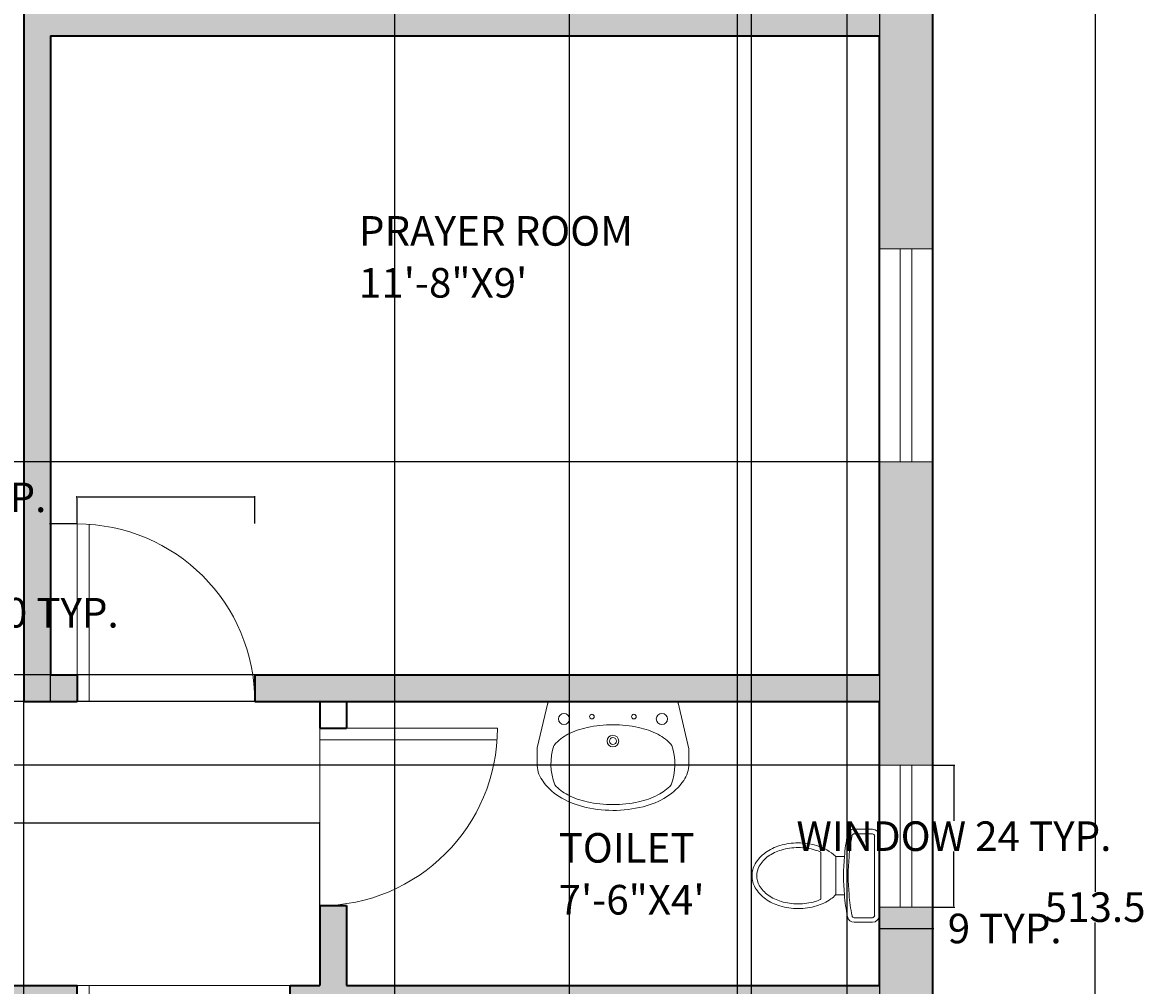
# Model space of a CAD drawing. Units: inches. Extents: x 2807 to 3326, y 2005 to 2580.
# Tile 11 of 12: x 3135 to 3325, y 2280 to 2442. Entities that reach past the tile are written whole.
import ezdxf

# ---------------------------------------------------------------- set-up
doc = ezdxf.new("R2010")
doc.units = ezdxf.units.IN
doc.header["$LTSCALE"] = 0.4
for name, color, linetype, lineweight in [('A-ANNO-DIMS', 2, 'Continuous', 18), ('A-AREA-IDEN', 5, 'Continuous', 18), ('A-FLOR-FIXT', 8, 'Continuous', 18), ('A-WALL-PATT', 231, 'Continuous', 13), ('DOORS', 144, 'Continuous', 18), ('WALL', 233, 'Continuous', 35), ('WINDOWS', 132, 'Continuous', 18)]:
    doc.layers.add(name, color=color, linetype=linetype, lineweight=lineweight)
doc.styles.get("Standard").update_dxf_attribs({"font": 'txt', "height": 5})
doc.dimstyles.get("Standard").update_dxf_attribs({"dimtxt": 0.18, "dimasz": 0.18, "dimexe": 0.18, "dimexo": 0.0625, "dimgap": 0.09, "dimtad": 0, "dimtih": 1, "dimtoh": 1, "dimdec": 4, "dimzin": 0, "dimdsep": 46, "dimtxsty": 'Standard', "dimcen": 0.09, "dimadec": 0, "dimazin": 0, "dimtfac": 1, "dimtdec": 4, "dimtofl": 0, "dimtmove": 0, "dimatfit": 3, "dimfxl": 1, "dimtolj": 1, "dimtzin": 0, "dimarcsym": 0})

# ---------------------------------------------------------------- blocks, each defined once
blk = doc.blocks.new('WIN-36')
at = {"ltscale": 0.4}
for p, q in [((0, 36), (0, 0)), ((9, 36), (0, 36)), ((3.5, 36), (3.5, 0)), ((5.5, 36), (5.5, 0)), ((9, 0), (9, 36)), ((0, 0), (9, 0))]:
    blk.add_line(p, q, dxfattribs=at)
blk = doc.blocks.new('WIN-24')
at = {"ltscale": 0.4}
for p, q in [((0, 0), (-9, 0)), ((-9, 0), (-9, -24)), ((-5.5, -24), (-5.5, 0)), ((-3.5, -24), (-3.5, 0)), ((0, -24), (0, 0)), ((-9, -24), (0, -24))]:
    blk.add_line(p, q, dxfattribs=at)
blk = doc.blocks.new('DOOR-30')
for p, q in [((0, 0), (-30, 0)), ((-2, -29.93), (-2, 0)), ((0, -30), (0, 0))]:
    blk.add_line(p, q)
blk.add_arc((0, 0), 30, 180, 270)
blk = doc.blocks.new('DOOR-36')
for p, q in [((0, 0), (-36, 0)), ((-2, -35.94), (-2, 0)), ((0, -36), (0, 0))]:
    blk.add_line(p, q)
blk.add_arc((0, 0), 36, 180, 270)
blk = doc.blocks.new('WC')
for p, q in [((-1.18, 7.87), (-4.23, 7.87)), ((-1.18, 7.09), (-4.23, 7.09)), ((-0.79, -6.69), (-0.79, 6.69)), ((0, -6.69), (0, 6.69)), ((-9.87, -3.98), (-9.87, 3.98)), ((-7.37, -3.23), (-7.37, 3.26)), ((-7.37, 3.26), (-5.9, 3.26)), ((-7.37, -3.23), (-5.9, -3.23)), ((-4.23, -7.09), (-1.18, -7.09)), ((-4.23, -7.87), (-1.18, -7.87))]:
    blk.add_line(p, q)
for centre, radius, start, end in [((-4.23, 6.69), 1.18, 90, 169.2553), ((-1.18, 6.69), 1.18, 0, 90), ((31.04, 0), 37.08, 169.2553, 174.96), ((31.04, 0), 36.29, 169.2553, 174.96), ((-4.23, 6.69), 0.394, 90, 169.2553), ((-1.18, 6.69), 0.394, 0, 90), ((-15.68, -1.06), 6.11, 125.4032, 149.7669), ((-14.49, -2.74), 8.17, 106.4045, 125.4032), ((-14.49, -2.74), 7.39, 106.4045, 125.4032), ((-13.7, -5.39), 10.94, 90, 106.4045), ((-13.7, -5.39), 10.15, 90, 106.4045), ((-13.7, -5.39), 10.94, 73.5955, 90), ((-13.7, -5.39), 10.15, 73.5955, 90), ((-12.92, -2.74), 7.39, 65.5529, 73.5955), ((-12.92, -2.74), 8.17, 47.2276, 73.5955), ((-17.5, 0), 4, 149.7669, 180), ((-15.68, -1.06), 5.33, 125.4032, 149.7669), ((31.04, 0), 37.08, 174.96, 184.9899), ((31.04, 0), 36.29, 174.96, 184.9899), ((-17.5, 0), 3.21, 149.7669, 180), ((-17.5, 0), 4, 180, 210.2331), ((-17.5, 0), 3.21, 180, 210.2331), ((-15.68, 1.06), 5.33, 210.2331, 234.5968), ((-15.68, 1.06), 6.11, 210.2331, 234.5968), ((-14.49, 2.74), 7.39, 234.5968, 253.5955), ((-11.73, 1.06), 6.11, 305.4032, 315.4553), ((31.04, 0), 37.08, 184.9899, 190.7447), ((31.04, 0), 36.29, 184.9899, 190.7447), ((-14.49, 2.74), 8.17, 234.5968, 253.5955), ((-13.7, 5.39), 10.94, 253.5955, 270), ((-13.7, 5.39), 10.15, 253.5955, 270), ((-13.7, 5.39), 10.15, 270, 286.4045), ((-13.7, 5.39), 10.94, 270, 286.4045), ((-12.92, 2.74), 7.39, 286.4045, 294.4471), ((-12.92, 2.74), 8.17, 286.4045, 305.4032), ((-4.23, -6.69), 1.18, 190.7447, 270), ((-4.23, -6.69), 0.394, 190.7447, 270), ((-1.18, -6.69), 0.394, 270, 0), ((-1.18, -6.69), 1.18, 270, 0)]:
    blk.add_arc(centre, radius, start, end)
blk = doc.blocks.new('LAVATORY-WALL')
for p, q in [((-12.82, 8.02), (-12.82, 10.56)), ((12.82, 8.02), (12.82, 10.56)), ((-12.82, 8.02), (-11.02, 0.2)), ((12.82, 7.85), (11.02, 0.2)), ((9.76, 7.2), (9.85, 7.28)), ((9.86, 7.44), (9.86, 7.31)), ((-11.02, 0), (-11.02, 0.39)), ((11.02, 0), (-11.02, 0)), ((11.02, 0.39), (11.02, 0))]:
    blk.add_line(p, q)
for centre, radius in [((0, 6.69), 0.984), ((0, 6.69), 0.591), ((-8.27, 2.95), 0.945), ((8.27, 2.95), 0.945), ((8.27, 2.95), 0.945), ((8.27, 2.95), 0.945), ((-3.54, 2.56), 0.394), ((3.54, 2.56), 0.394)]:
    blk.add_circle(centre, radius)
for centre, radius, start, end in [((-1.65, 3.98), 14.22, 104.0583, 121.3573), ((-0.05, -2.38), 20.78, 89.7676, 104.0583), ((0, -3.48), 20.89, 90, 102.0046), ((0, -3.48), 20.89, 77.9954, 90), ((-0.05, -2.38), 20.78, 75.477, 89.7676), ((1.59, 3.97), 14.22, 58.1779, 75.477), ((-4.1, 8.01), 9.5, 121.3573, 145.8048), ((-4.07, 8.92), 7.73, 117.1742, 138.1444), ((-1.62, 4.13), 13.11, 102.0046, 117.1742), ((1.62, 4.13), 13.11, 62.8258, 77.9954), ((4.07, 8.92), 7.73, 41.9499, 62.8258), ((4.08, 7.98), 9.5, 33.7305, 58.1779), ((-7.83, 10.54), 4.99, 145.8048, 179.7676), ((-0.53, 10.56), 9.94, 159.3022, 198.4613), ((0.53, 10.56), 9.94, 341.5387, 20.6978), ((7.83, 10.48), 4.99, 359.7676, 33.7305), ((-7.83, 10.54), 4.99, 179.7676, 180.9606), ((7.83, 8.04), 4.99, 357.883, 359.7676), ((-4.07, 12.42), 7.73, 220.3901, 242.8258), ((4.07, 12.42), 7.73, 297.1742, 318.6261), ((9.82, 7.31), 0.0394, 311.3224, 0), ((-1.62, 17.21), 13.11, 242.8258, 257.9954), ((0, 24.82), 20.89, 257.9954, 270), ((0, 24.82), 20.89, 270, 282.0046), ((1.62, 17.21), 13.11, 282.0046, 297.1742)]:
    blk.add_arc(centre, radius, start, end)
at = {"width": 0.8, "flags": 9}
for tag in ['XSIZE', 'YSIZE']:
    blk.add_attdef(tag, (0, 0), '', height=0.0197, rotation=180, dxfattribs=at)
blk = doc.blocks.new('*D15')
at = {"layer": 'A-ANNO-DIMS', "color": 0, "lineweight": -2, "ltscale": 0.4, "transparency": 16777216}
for p, q in [((3288.63, 2316.82), (3292.35, 2316.82)), ((3292.17, 2316.64), (3292.17, 2307.41)), ((3292.17, 2293), (3292.17, 2302.23)), ((3288.63, 2292.82), (3292.35, 2292.82))]:
    blk.add_line(p, q, dxfattribs=at)
at = {"layer": 'A-ANNO-DIMS', "color": 0, "ltscale": 0.4, "transparency": 16777216}
for points in [[(3292.14, 2316.64), (3292.2, 2316.64), (3292.17, 2316.82)], [(3292.14, 2293), (3292.2, 2293), (3292.17, 2292.82)]]:
    blk.add_solid(points, dxfattribs=at)
at = {"layer": 'Defpoints', "color": 0, "ltscale": 0.4, "transparency": 16777216}
for p in [(3288.57, 2316.82), (3292.17, 2316.82), (3288.57, 2292.82)]:
    blk.add_point(p, dxfattribs=at)
at = {"layer": 'A-ANNO-DIMS', "color": 0, "ltscale": 0.4, "transparency": 16777216, "insert": (3292.17, 2304.82), "char_height": 5, "attachment_point": 5}
blk.add_mtext('\\A1;WINDOW 24 TYP.', dxfattribs=at)
blk = doc.blocks.new('*D16')
at = {"layer": 'A-ANNO-DIMS', "color": 0, "lineweight": -2, "ltscale": 0.4, "transparency": 16777216}
for p, q in [((3279.57, 2292.76), (3279.57, 2289.04)), ((3288.57, 2292.76), (3288.57, 2289.04)), ((3279.75, 2289.22), (3288.39, 2289.22)), ((3288.57, 2289.22), (3288.75, 2289.22))]:
    blk.add_line(p, q, dxfattribs=at)
at = {"layer": 'A-ANNO-DIMS', "color": 0, "ltscale": 0.4, "transparency": 16777216}
for points in [[(3279.75, 2289.25), (3279.75, 2289.19), (3279.57, 2289.22)], [(3288.39, 2289.25), (3288.39, 2289.19), (3288.57, 2289.22)]]:
    blk.add_solid(points, dxfattribs=at)
at = {"layer": 'Defpoints', "color": 0, "ltscale": 0.4, "transparency": 16777216}
for p in [(3279.57, 2292.82), (3288.57, 2292.82), (3288.57, 2289.22)]:
    blk.add_point(p, dxfattribs=at)
at = {"layer": 'A-ANNO-DIMS', "color": 0, "ltscale": 0.4, "transparency": 16777216, "insert": (3300.74, 2289.22), "char_height": 5, "attachment_point": 5}
blk.add_mtext('\\A1;9 TYP.', dxfattribs=at)
blk = doc.blocks.new('*D19')
at = {"layer": 'A-ANNO-DIMS', "color": 0, "lineweight": -2, "ltscale": 0.4, "transparency": 16777216}
for p, q in [((3144.07, 2362.08), (3143.89, 2362.08)), ((3144.07, 2357.64), (3144.07, 2362.26)), ((3173.89, 2362.08), (3144.25, 2362.08)), ((3174.07, 2357.64), (3174.07, 2362.26))]:
    blk.add_line(p, q, dxfattribs=at)
at = {"layer": 'A-ANNO-DIMS', "color": 0, "ltscale": 0.4, "transparency": 16777216}
for points in [[(3144.25, 2362.11), (3144.25, 2362.05), (3144.07, 2362.08)], [(3173.89, 2362.11), (3173.89, 2362.05), (3174.07, 2362.08)]]:
    blk.add_solid(points, dxfattribs=at)
at = {"layer": 'Defpoints', "color": 0, "ltscale": 0.4, "transparency": 16777216}
for p in [(3144.07, 2362.08), (3144.07, 2357.58), (3174.07, 2357.58)]:
    blk.add_point(p, dxfattribs=at)
at = {"layer": 'A-ANNO-DIMS', "color": 0, "ltscale": 0.4, "transparency": 16777216, "insert": (3117.01, 2362.08), "char_height": 5, "attachment_point": 5}
blk.add_mtext('\\A1;DOOR 30 TYP.', dxfattribs=at)
blk = doc.blocks.new('*D20')
at = {"layer": 'A-ANNO-DIMS', "color": 0, "lineweight": -2, "ltscale": 0.4, "transparency": 16777216}
for p, q in [((3144, 2357.58), (3139.39, 2357.58)), ((3139.57, 2357.4), (3139.57, 2345.17)), ((3139.57, 2327.76), (3139.57, 2339.99)), ((3144, 2327.58), (3139.39, 2327.58))]:
    blk.add_line(p, q, dxfattribs=at)
at = {"layer": 'A-ANNO-DIMS', "color": 0, "ltscale": 0.4, "transparency": 16777216}
for points in [[(3139.54, 2357.4), (3139.6, 2357.4), (3139.57, 2357.58)], [(3139.54, 2327.76), (3139.6, 2327.76), (3139.57, 2327.58)]]:
    blk.add_solid(points, dxfattribs=at)
at = {"layer": 'Defpoints', "color": 0, "ltscale": 0.4, "transparency": 16777216}
for p in [(3144.07, 2357.58), (3139.57, 2327.58), (3144.07, 2327.58)]:
    blk.add_point(p, dxfattribs=at)
at = {"layer": 'A-ANNO-DIMS', "color": 0, "ltscale": 0.4, "transparency": 16777216, "insert": (3139.57, 2342.58), "char_height": 5, "attachment_point": 5}
blk.add_mtext('\\A1;30 TYP.', dxfattribs=at)
blk = doc.blocks.new('*D32')
at = {"layer": 'A-ANNO-DIMS', "color": 0, "lineweight": -2, "ltscale": 0.4, "transparency": 16777216}
for p, q in [((3288.629691, 2549.576496), (3316.197191, 2549.576496)), ((3316.017191, 2549.396496), (3316.017191, 2295.416496)), ((3316.017191, 2036.256496), (3316.017191, 2290.236496)), ((3148.629691, 2036.076496), (3316.197191, 2036.076496))]:
    blk.add_line(p, q, dxfattribs=at)
at = {"layer": 'A-ANNO-DIMS', "color": 0, "ltscale": 0.4, "transparency": 16777216}
for points in [[(3315.987191, 2549.396496), (3316.047191, 2549.396496), (3316.017191, 2549.576496)], [(3315.987191, 2036.256496), (3316.047191, 2036.256496), (3316.017191, 2036.076496)]]:
    blk.add_solid(points, dxfattribs=at)
at = {"layer": 'Defpoints', "color": 0, "ltscale": 0.4, "transparency": 16777216}
for p in [(3288.567191, 2549.576496), (3316.017191, 2549.576496), (3148.567191, 2036.076496)]:
    blk.add_point(p, dxfattribs=at)
at = {"layer": 'A-ANNO-DIMS', "color": 0, "ltscale": 0.4, "transparency": 16777216, "insert": (3316.017191, 2292.826496), "char_height": 5, "attachment_point": 5}
blk.add_mtext('\\A1;513.5', dxfattribs=at)
blk = doc.blocks.new('*D46')
at = {"layer": 'A-ANNO-DIMS', "color": 0, "lineweight": -2, "ltscale": 0.4, "transparency": 16777216}
for p, q in [((3279.5, 2327.58), (2816.94, 2327.58)), ((2817.12, 2327.4), (2817.12, 2324.79)), ((2817.12, 2317), (2817.12, 2319.61)), ((3279.5, 2316.82), (2816.94, 2316.82))]:
    blk.add_line(p, q, dxfattribs=at)
at = {"layer": 'A-ANNO-DIMS', "color": 0, "ltscale": 0.4, "transparency": 16777216}
for points in [[(2817.09, 2327.4), (2817.15, 2327.4), (2817.12, 2327.58)], [(2817.09, 2317), (2817.15, 2317), (2817.12, 2316.82)]]:
    blk.add_solid(points, dxfattribs=at)
at = {"layer": 'Defpoints', "color": 0, "ltscale": 0.4, "transparency": 16777216}
for p in [(2817.12, 2327.58), (3279.57, 2327.58), (3279.57, 2316.82)]:
    blk.add_point(p, dxfattribs=at)
at = {"layer": 'A-ANNO-DIMS', "color": 0, "ltscale": 0.4, "transparency": 16777216, "insert": (2817.12, 2322.2), "char_height": 5, "attachment_point": 5}
blk.add_mtext('\\A1;10.754', dxfattribs=at)
blk = doc.blocks.new('*D47')
at = {"layer": 'A-ANNO-DIMS', "color": 0, "lineweight": -2, "ltscale": 0.4, "transparency": 16777216}
for p, q in [((3279.504691, 2368.076496), (2816.937191, 2368.076496)), ((2817.117191, 2367.896496), (2817.117191, 2352.666496)), ((2817.117191, 2332.256496), (2817.117191, 2347.486496)), ((3279.504691, 2332.076496), (2816.937191, 2332.076496))]:
    blk.add_line(p, q, dxfattribs=at)
at = {"layer": 'A-ANNO-DIMS', "color": 0, "ltscale": 0.4, "transparency": 16777216}
for points in [[(2817.087191, 2367.896496), (2817.147191, 2367.896496), (2817.117191, 2368.076496)], [(2817.087191, 2332.256496), (2817.147191, 2332.256496), (2817.117191, 2332.076496)]]:
    blk.add_solid(points, dxfattribs=at)
at = {"layer": 'Defpoints', "color": 0, "ltscale": 0.4, "transparency": 16777216}
for p in [(2817.117191, 2368.076496), (3279.567191, 2368.076496), (3279.567191, 2332.076496)]:
    blk.add_point(p, dxfattribs=at)
at = {"layer": 'A-ANNO-DIMS', "color": 0, "ltscale": 0.4, "transparency": 16777216, "insert": (2817.117191, 2350.076496), "char_height": 5, "attachment_point": 5}
blk.add_mtext('\\A1;36', dxfattribs=at)
blk = doc.blocks.new('*D49')
at = {"layer": 'A-ANNO-DIMS', "color": 0, "lineweight": -2, "ltscale": 0.4, "transparency": 16777216}
for p, q in [((3255.57, 2444.51), (3255.57, 2008.45)), ((3279.57, 2444.51), (3279.57, 2008.45)), ((3255.75, 2008.63), (3263.31, 2008.63)), ((3279.39, 2008.63), (3271.82, 2008.63))]:
    blk.add_line(p, q, dxfattribs=at)
at = {"layer": 'A-ANNO-DIMS', "color": 0, "ltscale": 0.4, "transparency": 16777216}
for points in [[(3255.75, 2008.66), (3255.75, 2008.6), (3255.57, 2008.63)], [(3279.39, 2008.66), (3279.39, 2008.6), (3279.57, 2008.63)]]:
    blk.add_solid(points, dxfattribs=at)
at = {"layer": 'Defpoints', "color": 0, "ltscale": 0.4, "transparency": 16777216}
for p in [(3255.57, 2444.58), (3279.57, 2444.58), (3279.57, 2008.63)]:
    blk.add_point(p, dxfattribs=at)
at = {"layer": 'A-ANNO-DIMS', "color": 0, "ltscale": 0.4, "transparency": 16777216, "insert": (3267.57, 2008.63), "char_height": 5, "attachment_point": 5}
blk.add_mtext('\\A1;24', dxfattribs=at)
blk = doc.blocks.new('*D53')
at = {"layer": 'A-ANNO-DIMS', "color": 0, "lineweight": -2, "ltscale": 0.4, "transparency": 16777216}
for p, q in [((3197.668377, 2520.617027), (3197.668377, 2008.446496)), ((3227.195877, 2520.617027), (3227.195877, 2008.446496)), ((3197.848377, 2008.626496), (3202.342127, 2008.626496)), ((3227.015877, 2008.626496), (3222.522127, 2008.626496))]:
    blk.add_line(p, q, dxfattribs=at)
at = {"layer": 'A-ANNO-DIMS', "color": 0, "ltscale": 0.4, "transparency": 16777216}
for points in [[(3197.848377, 2008.656496), (3197.848377, 2008.596496), (3197.668377, 2008.626496)], [(3227.015877, 2008.656496), (3227.015877, 2008.596496), (3227.195877, 2008.626496)]]:
    blk.add_solid(points, dxfattribs=at)
at = {"layer": 'Defpoints', "color": 0, "ltscale": 0.4, "transparency": 16777216}
for p in [(3197.668377, 2520.679527), (3227.195877, 2520.679527), (3227.195877, 2008.626496)]:
    blk.add_point(p, dxfattribs=at)
at = {"layer": 'A-ANNO-DIMS', "color": 0, "ltscale": 0.4, "transparency": 16777216, "insert": (3212.432127, 2008.626496), "char_height": 5, "attachment_point": 5}
blk.add_mtext('\\A1;29.53', dxfattribs=at)
blk = doc.blocks.new('*D55')
at = {"layer": 'A-ANNO-DIMS', "color": 0, "lineweight": -2, "ltscale": 0.4, "transparency": 16777216}
for p, q in [((3257.92, 2460.31), (3257.92, 2008.45)), ((3274.06, 2460.31), (3274.06, 2008.45)), ((3258.1, 2008.63), (3273.88, 2008.63)), ((3274.06, 2008.63), (3274.24, 2008.63))]:
    blk.add_line(p, q, dxfattribs=at)
at = {"layer": 'A-ANNO-DIMS', "color": 0, "ltscale": 0.4, "transparency": 16777216}
for points in [[(3258.1, 2008.66), (3258.1, 2008.6), (3257.92, 2008.63)], [(3273.88, 2008.66), (3273.88, 2008.6), (3274.06, 2008.63)]]:
    blk.add_solid(points, dxfattribs=at)
at = {"layer": 'Defpoints', "color": 0, "ltscale": 0.4, "transparency": 16777216}
for p in [(3257.92, 2460.37), (3274.06, 2460.37), (3274.06, 2008.63)]:
    blk.add_point(p, dxfattribs=at)
at = {"layer": 'A-ANNO-DIMS', "color": 0, "ltscale": 0.4, "transparency": 16777216, "insert": (3285.76, 2008.63), "char_height": 5, "attachment_point": 5}
blk.add_mtext('\\A1;16.142', dxfattribs=at)
blk = doc.blocks.new('*D66')
at = {"layer": 'A-ANNO-DIMS', "color": 0, "lineweight": -2, "ltscale": 0.4, "transparency": 16777216}
for p, q in [((3129.534988, 2263.581941), (3129.534988, 2577.206496)), ((3129.714988, 2577.026496), (3134.887191, 2577.026496)), ((3135.067191, 2275.138996), (3135.067191, 2577.206496)), ((3135.067191, 2577.026496), (3135.247191, 2577.026496))]:
    blk.add_line(p, q, dxfattribs=at)
at = {"layer": 'A-ANNO-DIMS', "color": 0, "ltscale": 0.4, "transparency": 16777216}
for points in [[(3129.714988, 2577.056496), (3129.714988, 2576.996496), (3129.534988, 2577.026496)], [(3134.887191, 2577.056496), (3134.887191, 2576.996496), (3135.067191, 2577.026496)]]:
    blk.add_solid(points, dxfattribs=at)
at = {"layer": 'Defpoints', "color": 0, "ltscale": 0.4, "transparency": 16777216}
for p in [(3135.067191, 2577.026496), (3135.067191, 2275.076496), (3129.534988, 2263.519441)]:
    blk.add_point(p, dxfattribs=at)
at = {"layer": 'A-ANNO-DIMS', "color": 0, "ltscale": 0.4, "transparency": 16777216, "insert": (3145.337191, 2577.026496), "char_height": 5, "attachment_point": 5}
blk.add_mtext('\\A1;5.532', dxfattribs=at)
blk = doc.blocks.new('*D72')
at = {"layer": 'A-ANNO-DIMS', "color": 0, "lineweight": -2, "ltscale": 0.4, "transparency": 16777216}
for p, q in [((2948.07, 2279.64), (2948.07, 2307.21)), ((2948.25, 2307.03), (3060.05, 2307.03)), ((3184.89, 2307.03), (3073.09, 2307.03)), ((3185.07, 2279.64), (3185.07, 2307.21))]:
    blk.add_line(p, q, dxfattribs=at)
at = {"layer": 'A-ANNO-DIMS', "color": 0, "ltscale": 0.4, "transparency": 16777216}
for points in [[(2948.25, 2307.06), (2948.25, 2307), (2948.07, 2307.03)], [(3184.89, 2307.06), (3184.89, 2307), (3185.07, 2307.03)]]:
    blk.add_solid(points, dxfattribs=at)
at = {"layer": 'Defpoints', "color": 0, "ltscale": 0.4, "transparency": 16777216}
for p in [(3185.07, 2307.03), (2948.07, 2279.58), (3185.07, 2279.58)]:
    blk.add_point(p, dxfattribs=at)
at = {"layer": 'A-ANNO-DIMS', "color": 0, "ltscale": 0.4, "transparency": 16777216, "insert": (3066.57, 2307.03), "char_height": 5, "attachment_point": 5}
blk.add_mtext('\\A1;237', dxfattribs=at)

msp = doc.modelspace()

# ---------------------------------------------------------------- hatches: boundary and pattern name
at = {"layer": 'A-WALL-PATT', "ltscale": 0.4}
h = msp.add_hatch(color=256, dxfattribs=at)
h.dxf.hatch_style = 1
h.paths.add_polyline_path([(3288.5672, 2549.5765), (2941.5672, 2549.5765), (2941.5672, 2540.5765), (2993.5672, 2540.5765), (2993.5672, 2489.5693), (2998.0672, 2489.5693), (2998.0672, 2540.5765), (3135.0672, 2540.5765), (3135.0672, 2479.0765), (3139.5672, 2479.0765), (3139.5672, 2540.5765), (3279.5672, 2540.5765), (3279.5672, 2510.5765), (3288.5672, 2510.5765)])
h.paths.add_polyline_path([(2905.5672, 2549.5765), (2844.5672, 2549.5765), (2844.5672, 2445.94), (2853.5672, 2445.94), (2853.5672, 2540.5765), (2905.5672, 2540.5765)])
h.paths.add_polyline_path([(2853.5672, 2409.94), (2844.5672, 2409.94), (2844.5672, 2371.3497), (2853.5672, 2371.3497), (2853.5672, 2380.0765), (2909.0672, 2380.0765), (2909.0672, 2384.5765), (2853.5672, 2384.5765)])
h.paths.add_polyline_path([(2998.0672, 2389.0765), (2993.5672, 2389.0765), (2993.5672, 2384.5765), (2939.0672, 2384.5765), (2939.0672, 2380.0765), (2943.5672, 2380.0765), (2943.5672, 2314.0765), (2948.0672, 2314.0765), (2948.0672, 2380.0765), (2998.0672, 2380.0765)])
h.paths.add_polyline_path([(2998.0672, 2471.8029), (2993.5672, 2471.8029), (2993.5672, 2425.0765), (2998.0672, 2425.0765)])
h.paths.add_polyline_path([(2953.0672, 2279.5765), (2948.0672, 2279.5765), (2948.0672, 2284.0765), (2943.5672, 2284.0765), (2943.5672, 2279.5765), (2853.5672, 2279.5765), (2853.5672, 2289.0663), (2844.5672, 2289.0663), (2844.5672, 2227.8961), (2853.5672, 2227.8961), (2853.5672, 2275.0765), (2953.0672, 2275.0765)])
h.paths.add_polyline_path([(2943.5672, 2332.0765), (2853.5672, 2332.0765), (2853.5672, 2347.3497), (2844.5672, 2347.3497), (2844.5672, 2313.0663), (2853.5672, 2313.0663), (2853.5672, 2327.5765), (2943.5672, 2327.5765)])
h.paths.add_polyline_path([(3144.0672, 2279.5765), (2993.5672, 2279.5765), (2989.0672, 2279.5765), (2989.0672, 2275.0765), (2993.5672, 2275.0765), (2993.5672, 2144.5765), (2984.5672, 2144.5765), (2984.5672, 2135.5765), (2993.5672, 2135.5765), (2993.5672, 2120.0765), (3036.5672, 2120.0765), (3036.5672, 2129.0765), (2998.0672, 2129.0765), (2998.0672, 2275.0765), (3135.0672, 2275.0765), (3135.0672, 2129.0765), (3096.5672, 2129.0765), (3096.5672, 2120.0765), (3139.5672, 2120.0765), (3139.5672, 2135.5765), (3148.5672, 2135.5765), (3148.5672, 2144.5765), (3139.5672, 2144.5765), (3139.5672, 2275.0765), (3144.0672, 2275.0765)])
h.paths.add_polyline_path([(2984.5672, 2144.5765), (2925.9914, 2144.5765), (2925.9914, 2135.5765), (2984.5672, 2135.5765)])
h.paths.add_polyline_path([(2889.9914, 2144.5765), (2853.5672, 2144.5765), (2853.5672, 2191.8961), (2844.5672, 2191.8961), (2844.5672, 2135.5765), (2889.9914, 2135.5765)])
h.paths.add_polyline_path([(3196.0672, 2144.5765), (3148.5672, 2144.5765), (3148.5672, 2135.5765), (3196.0672, 2135.5765)])
h.paths.add_polyline_path([(3288.5672, 2191.8265), (3279.5672, 2191.8265), (3279.5672, 2144.5765), (3232.0672, 2144.5765), (3232.0672, 2135.5765), (3288.5672, 2135.5765)])
h.paths.add_polyline_path([(3288.5672, 2292.8229), (3279.5672, 2292.8229), (3279.5672, 2291.4371), (3279.5672, 2279.5765), (3189.5672, 2279.5765), (3189.5672, 2293.0765), (3185.0672, 2293.0765), (3185.0672, 2279.5765), (3180.0672, 2279.5765), (3180.0672, 2275.0765), (3279.5672, 2275.0765), (3279.5672, 2227.8265), (3288.5672, 2227.8265)])
h.paths.add_polyline_path([(3288.5672, 2368.0765), (3279.5672, 2368.0765), (3279.5672, 2332.0765), (3174.0672, 2332.0765), (3174.0672, 2327.5765), (3185.0672, 2327.5765), (3189.5672, 2327.5765), (3279.5672, 2327.5765), (3279.5672, 2316.8229), (3288.5672, 2316.8229)])
h.paths.add_polyline_path([(3288.5672, 2474.5765), (3279.5672, 2474.5765), (3279.5672, 2444.5765), (3139.5672, 2444.5765), (3139.5672, 2449.0765), (3135.0672, 2449.0765), (3135.0672, 2327.5765), (3144.0672, 2327.5765), (3144.0672, 2332.0765), (3139.5672, 2332.0765), (3139.5672, 2440.0765), (3279.5672, 2440.0765), (3279.5672, 2404.0765), (3288.5672, 2404.0765)])

# ---------------------------------------------------------------- linework, layer by layer
at = {"layer": 'WALL'}
for p, q in [((3288.5672, 2549.5765), (3288.5672, 2135.5765)), ((3135.0672, 2449.0765), (3135.0672, 2327.5765)), ((3139.5672, 2440.0765), (3279.5672, 2440.0765)), ((3139.5672, 2440.0765), (3139.5672, 2332.0765)), ((3279.5672, 2440.0765), (3279.5672, 2332.0765)), ((3139.5672, 2332.0765), (3144.0672, 2332.0765)), ((3144.0672, 2332.0765), (3144.0672, 2327.5765)), ((3174.0672, 2332.0765), (3174.0672, 2327.5765)), ((3174.0672, 2332.0765), (3279.5672, 2332.0765)), ((3135.0672, 2327.5765), (3144.0672, 2327.5765)), ((3174.0672, 2327.5765), (3185.0672, 2327.5765)), ((3185.0672, 2327.5765), (3185.0672, 2323.0765)), ((3185.0672, 2327.5765), (3189.5672, 2327.5765)), ((3189.5672, 2327.5765), (3189.5672, 2323.0765)), ((3189.5672, 2327.5765), (3279.5672, 2327.5765)), ((3279.5672, 2327.5765), (3279.5672, 2279.5765)), ((3185.0672, 2323.0765), (3189.5672, 2323.0765)), ((3185.0672, 2293.0765), (3189.5672, 2293.0765)), ((3185.0672, 2293.0765), (3185.0672, 2279.5765)), ((3189.5672, 2293.0765), (3189.5672, 2279.5765)), ((2993.5672, 2279.5765), (3144.0672, 2279.5765)), ((3144.0672, 2275.0765), (3144.0672, 2279.5765)), ((3180.0672, 2275.0765), (3180.0672, 2279.5765)), ((3180.0672, 2279.5765), (3185.0672, 2279.5765)), ((3189.5672, 2279.5765), (3279.5672, 2279.5765))]:
    msp.add_line(p, q, dxfattribs=at)

# ---------------------------------------------------------------- block references
at = {"layer": 'A-FLOR-FIXT', "rotation": 180}
msp.add_blockref('LAVATORY-WALL', (3234.5672, 2327.5765), dxfattribs=at)
at = {"layer": 'A-FLOR-FIXT'}
msp.add_blockref('WC', (3279.567, 2298.13), dxfattribs=at)
at = {"layer": 'DOORS'}
for p, rotation in [((3144.0672, 2327.5765), 180), ((3185.0672, 2323.0765), 89.99999999999945)]:
    msp.add_blockref('DOOR-30', p, dxfattribs=dict(at, rotation=rotation))
at = {"layer": 'DOORS', "extrusion": (0, 0, -1), "zscale": -1}
msp.add_blockref('DOOR-36', (-3144.0672, 2279.5765), dxfattribs=at)
at = {"layer": 'WINDOWS'}
for name, p in [('WIN-36', (3279.5672, 2368.0765)), ('WIN-24', (3288.5672, 2316.8229))]:
    msp.add_blockref(name, p, dxfattribs=at)

# ---------------------------------------------------------------- texts
at = {"layer": 'A-AREA-IDEN', "ltscale": 0.4}
for s, p in [('PRAYER ROOM', (3191.659, 2404.6024)), ('11\'-8"X9\'', (3191.659, 2395.8285)), ('TOILET', (3225.395, 2300.35)), ('7\'-6"X4\'', (3225.395, 2291.5761))]:
    msp.add_text(s, height=5, dxfattribs=at).set_placement(p)

# ---------------------------------------------------------------- dimensions: what is measured, and where the dimension line sits
at = {"layer": 'A-ANNO-DIMS', "ltscale": 0.4}
for base, p1, p2, override, picture, middle in [((3135.0672, 2577.0265), (3129.535, 2263.5194), (3135.0672, 2275.0765), {"dimdec": 3, "dimlfac": 1, "dimrnd": 0, "dimzin": 0, "dimdsep": 46, "dimlunit": 2}, '*D66', (3145.3372, 2577.0265)), ((3227.1959, 2008.6265), (3197.6684, 2520.6795), (3227.1959, 2520.6795), {"dimdec": 2, "dimlfac": 1, "dimrnd": 0, "dimzin": 0, "dimdsep": 46, "dimlunit": 2}, '*D53', (3212.4321, 2008.6265)), ((3274.0614, 2008.6265), (3257.9197, 2460.3683), (3274.0614, 2460.3683), {"dimdec": 3, "dimlfac": 1, "dimrnd": 0, "dimzin": 0, "dimdsep": 46, "dimlunit": 2}, '*D55', (3285.76, 2008.6265)), ((3279.5672, 2008.6265), (3255.5672, 2444.5765), (3279.5672, 2444.5765), {"dimdec": 0, "dimlfac": 1, "dimrnd": 0, "dimzin": 0, "dimdsep": 46, "dimlunit": 2}, '*D49', (3267.5672, 2008.6265))]:
    dim = msp.add_linear_dim(base=base, p1=p1, p2=p2, dimstyle='Standard', override=override, dxfattribs=at)
    dim.commit()
    dim.dimension.update_dxf_attribs({"geometry": picture, "text_midpoint": middle})
for base, p1, p2, angle, override, picture, middle in [((3316.0172, 2549.5765), (3148.5672, 2036.0765), (3288.5672, 2549.5765), 90, {"dimdec": 1, "dimlfac": 1, "dimrnd": 0, "dimzin": 0, "dimdsep": 46, "dimlunit": 2}, '*D32', (3316.0172, 2292.8265)), ((2817.1172, 2368.0765), (3279.5672, 2332.0765), (3279.5672, 2368.0765), 90, {"dimdec": 0, "dimlfac": 1, "dimrnd": 0, "dimzin": 0, "dimdsep": 46, "dimlunit": 2}, '*D47', (2817.1172, 2350.0765)), ((2817.1172, 2327.5765), (3279.5672, 2316.8229), (3279.5672, 2327.5765), 90, {"dimdec": 3, "dimlfac": 1, "dimrnd": 0, "dimzin": 0, "dimdsep": 46, "dimlunit": 2}, '*D46', (2817.1172, 2322.1997)), ((3185.0672, 2307.0265), (2948.0672, 2279.5765), (3185.0672, 2279.5765), 0, {"dimdec": 0, "dimlfac": 1, "dimrnd": 0, "dimzin": 0, "dimdsep": 46, "dimlunit": 2}, '*D72', (3066.5672, 2307.0265))]:
    dim = msp.add_linear_dim(base=base, p1=p1, p2=p2, angle=angle, dimstyle='Standard', override=override, dxfattribs=at)
    dim.commit()
    dim.dimension.update_dxf_attribs({"geometry": picture, "text_midpoint": middle})
for base, p1, p2, angle, text, picture, middle in [((3144.0672, 2362.0765), (3174.0672, 2357.5765), (3144.0672, 2357.5765), 180, 'DOOR <> TYP.', '*D19', (3117.0115, 2362.0765)), ((3139.5672, 2327.5765), (3144.0672, 2357.5765), (3144.0672, 2327.5765), 270, '<> TYP.', '*D20', (3139.5672, 2342.5765)), ((3292.1672, 2316.8229), (3288.5672, 2292.8229), (3288.5672, 2316.8229), 90, 'WINDOW <> TYP.', '*D15', (3292.1672, 2304.8229))]:
    dim = msp.add_linear_dim(base=base, p1=p1, p2=p2, angle=angle, text=text, dimstyle='Standard', override={"dimdec": 0, "dimlfac": 1, "dimrnd": 0, "dimzin": 0, "dimdsep": 46, "dimlunit": 2}, dxfattribs=at)
    dim.commit()
    dim.dimension.update_dxf_attribs({"geometry": picture, "text_midpoint": middle})
dim = msp.add_linear_dim(base=(3288.5672, 2289.2229), p1=(3279.5672, 2292.8229), p2=(3288.5672, 2292.8229), text='<> TYP.', dimstyle='Standard', override={"dimdec": 0, "dimlfac": 1, "dimrnd": 0, "dimzin": 0, "dimdsep": 46, "dimlunit": 2}, dxfattribs=at)
dim.commit()
dim.dimension.update_dxf_attribs({"geometry": '*D16', "text_midpoint": (3300.742, 2289.2229)})

doc.saveas('drawing.dxf')
